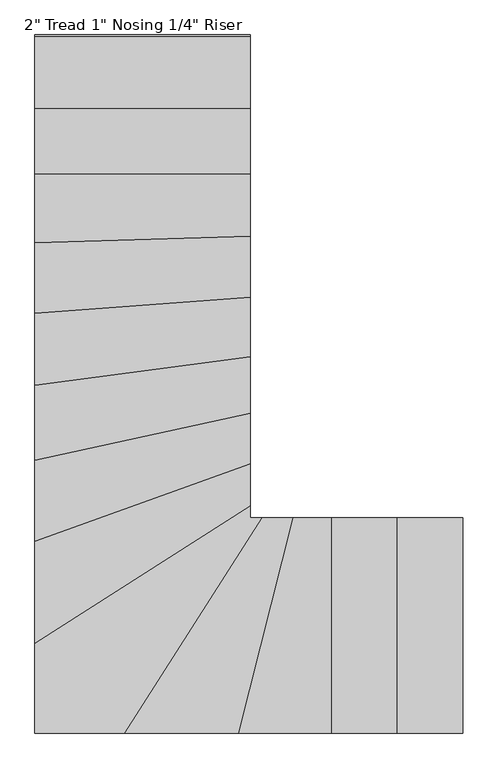
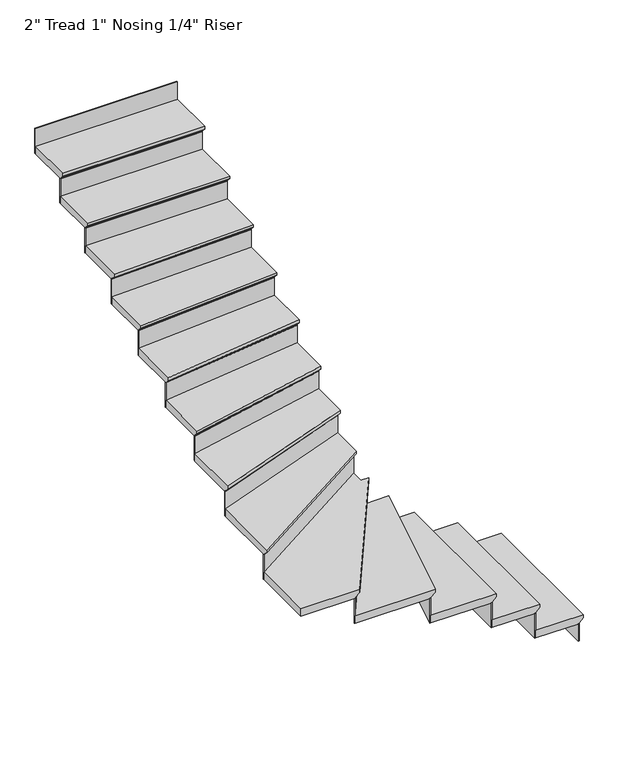
"""IFC4 building model written with IfcOpenShell, lengths in millimetres: stair flight geometry."""

from ifc_helpers import new_model, si_unit, origin, place, context, project, spatial, faceted_brep, source, transform, mapped, element, save


def stair_flight_d75d4b7d(model_context):
    return source(origin(), model_context, "Body", "Brep", [
        faceted_brep([(-4378.4230036, -1246.1564015, 4028.0166667), (-4378.4230036, -1246.1564015, 4047.0666667), (-4378.4230036, -2160.5564015, 4047.0666667), (-4378.4230036, -2160.5564015, 4028.0166667), (-4403.8230036, -1246.1564015, 4002.6166667), (-4403.8230036, -2160.5564015, 4002.6166667), (-4683.2230036, -1246.1564015, 4047.0666667), (-4683.2230036, -2160.5564015, 4047.0666667), (-4403.8230036, -2160.5564015, 3996.2666667), (-4683.2230036, -2160.5564015, 3996.2666667), (-4683.2230036, -1246.1564015, 3996.2666667), (-4403.8230036, -1246.1564015, 3996.2666667)], [[[0, 1, 2, 3]], [[4, 0, 3, 5]], [[2, 1, 6, 7]], [[8, 9, 10, 11]], [[2, 7, 9, 8, 5, 3]], [[8, 11, 4, 5]], [[6, 1, 0, 4, 11, 10]], [[7, 6, 10, 9]]]),
        faceted_brep([(-4403.8230036, -1246.1564015, 3996.2666667), (-4403.8230036, -1246.1564015, 3877.7333333), (-4410.1730036, -1246.1564015, 3877.7333333), (-4410.1730036, -1246.1564015, 3996.2666667), (-4403.8230036, -2160.5564015, 3996.2666667), (-4410.1730036, -2160.5564015, 3996.2666667), (-4410.1730036, -2160.5564015, 3877.7333333), (-4403.8230036, -2160.5564015, 3877.7333333)], [[[0, 1, 2, 3]], [[4, 5, 6, 7]], [[1, 0, 4, 7]], [[2, 1, 7, 6]], [[3, 2, 6, 5]], [[0, 3, 5, 4]]]),
        faceted_brep([(-4683.2230036, -1246.1564015, 4165.6), (-4683.2230036, -1246.1564015, 3996.2666667), (-4689.5730036, -1246.1564015, 3996.2666667), (-4689.5730036, -1246.1564015, 4165.6), (-4683.2230036, -2160.5564015, 4165.6), (-4689.5730036, -2160.5564015, 4165.6), (-4689.5730036, -2160.5564015, 3996.2666667), (-4683.2230036, -2160.5564015, 3996.2666667)], [[[0, 1, 2, 3]], [[4, 5, 6, 7]], [[1, 0, 4, 7]], [[2, 1, 7, 6]], [[3, 2, 6, 5]], [[0, 3, 5, 4]]]),
        faceted_brep([(-4657.8230036, -2160.5564015, 4216.4), (-4657.8230036, -1246.1564015, 4216.4), (-4962.6230036, -1246.1564015, 4216.4), (-4962.6230036, -2160.5564015, 4216.4), (-4683.2230036, -2160.5564015, 4165.6), (-4962.6230036, -2160.5564015, 4165.6), (-4962.6230036, -1246.1564015, 4165.6), (-4683.2230036, -1246.1564015, 4165.6), (-4683.2230036, -2160.5564015, 4171.95), (-4657.8230036, -2160.5564015, 4197.35), (-4683.2230036, -1246.1564015, 4171.95), (-4657.8230036, -1246.1564015, 4197.35)], [[[0, 1, 2, 3]], [[4, 5, 6, 7]], [[0, 3, 5, 4, 8, 9]], [[4, 7, 10, 8]], [[2, 1, 11, 10, 7, 6]], [[3, 2, 6, 5]], [[11, 1, 0, 9]], [[10, 11, 9, 8]]]),
        faceted_brep([(-4962.6230036, -1246.1564015, 4334.9333333), (-4962.6230036, -1246.1564015, 4165.6), (-4968.9730036, -1246.1564015, 4165.6), (-4968.9730036, -1246.1564015, 4334.9333333), (-4962.6230036, -2160.5564015, 4334.9333333), (-4968.9730036, -2160.5564015, 4334.9333333), (-4968.9730036, -2160.5564015, 4165.6), (-4962.6230036, -2160.5564015, 4165.6)], [[[0, 1, 2, 3]], [[4, 5, 6, 7]], [[1, 0, 4, 7]], [[2, 1, 7, 6]], [[3, 2, 6, 5]], [[0, 3, 5, 4]]]),
        faceted_brep([(-4937.2230036, -2160.5564015, 4385.7333333), (-4937.2230036, -1246.1564015, 4385.7333333), (-5127.3280374, -1246.1564015, 4385.7333333), (-5358.313714, -2160.5564015, 4385.7333333), (-4962.6230036, -2160.5564015, 4334.9333333), (-5358.313714, -2160.5564015, 4334.9333333), (-5127.3280374, -1246.1564015, 4334.9333333), (-4962.6230036, -1246.1564015, 4334.9333333), (-4962.6230036, -2160.5564015, 4341.2833333), (-4937.2230036, -2160.5564015, 4366.6833333), (-4962.6230036, -1246.1564015, 4341.2833333), (-4937.2230036, -1246.1564015, 4366.6833333)], [[[0, 1, 2, 3]], [[4, 5, 6, 7]], [[0, 3, 5, 4, 8, 9]], [[4, 7, 10, 8]], [[2, 1, 11, 10, 7, 6]], [[3, 2, 6, 5]], [[11, 1, 0, 9]], [[10, 11, 9, 8]]]),
        faceted_brep([(-5127.3280374, -1246.1564015, 4504.2666667), (-5127.3280374, -1246.1564015, 4334.9333333), (-5133.8775055, -1246.1564015, 4334.9333333), (-5133.8775055, -1246.1564015, 4504.2666667), (-5358.313714, -2160.5564015, 4504.2666667), (-5364.8631821, -2160.5564015, 4504.2666667), (-5364.8631821, -2160.5564015, 4334.9333333), (-5358.313714, -2160.5564015, 4334.9333333)], [[[0, 1, 2, 3]], [[4, 5, 6, 7]], [[1, 0, 4, 7]], [[2, 1, 7, 6]], [[3, 2, 6, 5]], [[0, 3, 5, 4]]]),
        faceted_brep([(-5332.1158419, -2160.5564015, 4555.0666667), (-5101.1301653, -1246.1564015, 4555.0666667), (-5261.5956265, -1246.1564015, 4555.0666667), (-5846.1950619, -2160.5564015, 4555.0666667), (-5358.313714, -2160.5564015, 4504.2666667), (-5846.1950619, -2160.5564015, 4504.2666667), (-5261.5956265, -1246.1564015, 4504.2666667), (-5127.3280374, -1246.1564015, 4504.2666667), (-5358.313714, -2160.5564015, 4510.6166667), (-5332.1158419, -2160.5564015, 4536.0166667), (-5127.3280374, -1246.1564015, 4510.6166667), (-5101.1301653, -1246.1564015, 4536.0166667)], [[[0, 1, 2, 3]], [[4, 5, 6, 7]], [[0, 3, 5, 4, 8, 9]], [[4, 7, 10, 8]], [[2, 1, 11, 10, 7, 6]], [[3, 2, 6, 5]], [[11, 1, 0, 9]], [[10, 11, 9, 8]]]),
        faceted_brep([(-5261.5956265, -1246.1564015, 4673.6), (-5261.5956265, -1246.1564015, 4504.2666667), (-5269.1324569, -1246.1564015, 4504.2666667), (-5269.1324569, -1246.1564015, 4673.6), (-5846.1950619, -2160.5564015, 4673.6), (-5853.7318923, -2160.5564015, 4673.6), (-5853.7318923, -2160.5564015, 4504.2666667), (-5846.1950619, -2160.5564015, 4504.2666667)], [[[0, 1, 2, 3]], [[4, 5, 6, 7]], [[1, 0, 4, 7]], [[2, 1, 7, 6]], [[3, 2, 6, 5]], [[0, 3, 5, 4]]]),
        faceted_brep([(-6196.7599931, -1749.696827, 4724.4), (-6196.7599931, -2160.5564015, 4724.4), (-5816.0477402, -2160.5564015, 4724.4), (-5231.4483048, -1246.1564015, 4724.4), (-5282.3599931, -1246.1564015, 4724.4), (-5282.3599931, -1165.0973916, 4724.4), (-6196.7599931, -2160.5564015, 4673.6), (-6196.7599931, -1749.696827, 4673.6), (-5282.3599931, -1165.0973916, 4673.6), (-5282.3599931, -1246.1564015, 4673.6), (-5261.5956265, -1246.1564015, 4673.6), (-5846.1950619, -2160.5564015, 4673.6), (-5261.5956265, -1246.1564015, 4679.95), (-5846.1950619, -2160.5564015, 4679.95), (-5231.4483048, -1246.1564015, 4705.35), (-5816.0477402, -2160.5564015, 4705.35)], [[[0, 1, 2, 3, 4, 5]], [[6, 7, 8, 9, 10, 11]], [[1, 0, 7, 6]], [[11, 10, 12, 13]], [[4, 3, 14, 12, 10, 9]], [[0, 5, 8, 7]], [[14, 3, 2, 15]], [[12, 14, 15, 13]], [[2, 1, 6, 11, 13, 15]], [[5, 4, 9, 8]]]),
        faceted_brep([(-5282.3599931, -1165.0973916, 4842.9333333), (-5282.3599931, -1165.0973916, 4673.6), (-5282.3599931, -1157.5605612, 4673.6), (-5282.3599931, -1157.5605612, 4842.9333333), (-6196.7599931, -1749.696827, 4842.9333333), (-6196.7599931, -1742.1599966, 4842.9333333), (-6196.7599931, -1742.1599966, 4673.6), (-6196.7599931, -1749.696827, 4673.6)], [[[0, 1, 2, 3]], [[4, 5, 6, 7]], [[1, 0, 4, 7]], [[2, 1, 7, 6]], [[3, 2, 6, 5]], [[0, 3, 5, 4]]]),
        faceted_brep([(-6196.7599931, -1779.8441487, 4893.7333333), (-5282.3599931, -1195.2447133, 4893.7333333), (-5282.3599931, -989.1410797, 4893.7333333), (-6196.7599931, -1317.7175845, 4893.7333333), (-6196.7599931, -1749.696827, 4842.9333333), (-6196.7599931, -1317.7175845, 4842.9333333), (-5282.3599931, -989.1410797, 4842.9333333), (-5282.3599931, -1165.0973916, 4842.9333333), (-6196.7599931, -1749.696827, 4849.2833333), (-6196.7599931, -1779.8441487, 4874.6833333), (-5282.3599931, -1165.0973916, 4849.2833333), (-5282.3599931, -1195.2447133, 4874.6833333)], [[[0, 1, 2, 3]], [[4, 5, 6, 7]], [[0, 3, 5, 4, 8, 9]], [[4, 7, 10, 8]], [[2, 1, 11, 10, 7, 6]], [[3, 2, 6, 5]], [[11, 1, 0, 9]], [[10, 11, 9, 8]]]),
        faceted_brep([(-5282.3599931, -989.1410797, 5012.2666667), (-5282.3599931, -989.1410797, 4842.9333333), (-5282.3599931, -982.3935597, 4842.9333333), (-5282.3599931, -982.3935597, 5012.2666667), (-6196.7599931, -1317.7175845, 5012.2666667), (-6196.7599931, -1310.9700645, 5012.2666667), (-6196.7599931, -1310.9700645, 4842.9333333), (-6196.7599931, -1317.7175845, 4842.9333333)], [[[0, 1, 2, 3]], [[4, 5, 6, 7]], [[1, 0, 4, 7]], [[2, 1, 7, 6]], [[3, 2, 6, 5]], [[0, 3, 5, 4]]]),
        faceted_brep([(-6196.7599931, -1344.7076644, 5063.0666667), (-5282.3599931, -1016.1311596, 5063.0666667), (-5282.3599931, -775.0246806, 5063.0666667), (-6196.7599931, -975.0133472, 5063.0666667), (-6196.7599931, -1317.7175845, 5012.2666667), (-6196.7599931, -975.0133472, 5012.2666667), (-5282.3599931, -775.0246806, 5012.2666667), (-5282.3599931, -989.1410797, 5012.2666667), (-6196.7599931, -1317.7175845, 5018.6166667), (-6196.7599931, -1344.7076644, 5044.0166667), (-5282.3599931, -989.1410797, 5018.6166667), (-5282.3599931, -1016.1311596, 5044.0166667)], [[[0, 1, 2, 3]], [[4, 5, 6, 7]], [[0, 3, 5, 4, 8, 9]], [[4, 7, 10, 8]], [[2, 1, 11, 10, 7, 6]], [[3, 2, 6, 5]], [[11, 1, 0, 9]], [[10, 11, 9, 8]]]),
        faceted_brep([(-5282.3599931, -775.0246806, 5181.6), (-5282.3599931, -775.0246806, 5012.2666667), (-5282.3599931, -768.5245811, 5012.2666667), (-5282.3599931, -768.5245811, 5181.6), (-6196.7599931, -975.0133472, 5181.6), (-6196.7599931, -968.5132477, 5181.6), (-6196.7599931, -968.5132477, 5012.2666667), (-6196.7599931, -975.0133472, 5012.2666667)], [[[0, 1, 2, 3]], [[4, 5, 6, 7]], [[1, 0, 4, 7]], [[2, 1, 7, 6]], [[3, 2, 6, 5]], [[0, 3, 5, 4]]]),
        faceted_brep([(-6196.7599931, -1001.0137453, 5232.4), (-5282.3599931, -801.0250787, 5232.4), (-5282.3599931, -535.4776405, 5232.4), (-6196.7599931, -656.5180526, 5232.4), (-6196.7599931, -975.0133472, 5181.6), (-6196.7599931, -656.5180526, 5181.6), (-5282.3599931, -535.4776405, 5181.6), (-5282.3599931, -775.0246806, 5181.6), (-6196.7599931, -975.0133472, 5187.95), (-6196.7599931, -1001.0137453, 5213.35), (-5282.3599931, -775.0246806, 5187.95), (-5282.3599931, -801.0250787, 5213.35)], [[[0, 1, 2, 3]], [[4, 5, 6, 7]], [[0, 3, 5, 4, 8, 9]], [[4, 7, 10, 8]], [[2, 1, 11, 10, 7, 6]], [[3, 2, 6, 5]], [[11, 1, 0, 9]], [[10, 11, 9, 8]]]),
        faceted_brep([(-5282.3599931, -535.4776405, 5350.9333333), (-5282.3599931, -535.4776405, 5181.6), (-5282.3599931, -529.0722492, 5181.6), (-5282.3599931, -529.0722492, 5350.9333333), (-6196.7599931, -656.5180526, 5350.9333333), (-6196.7599931, -650.1126613, 5350.9333333), (-6196.7599931, -650.1126613, 5181.6), (-6196.7599931, -656.5180526, 5181.6)], [[[0, 1, 2, 3]], [[4, 5, 6, 7]], [[1, 0, 4, 7]], [[2, 1, 7, 6]], [[3, 2, 6, 5]], [[0, 3, 5, 4]]]),
        faceted_brep([(-6196.7599931, -682.139618, 5401.7333333), (-5282.3599931, -561.099206, 5401.7333333), (-5282.3599931, -282.9309158, 5401.7333333), (-6196.7599931, -350.56912, 5401.7333333), (-6196.7599931, -656.5180526, 5350.9333333), (-6196.7599931, -350.56912, 5350.9333333), (-5282.3599931, -282.9309158, 5350.9333333), (-5282.3599931, -535.4776405, 5350.9333333), (-6196.7599931, -656.5180526, 5357.2833333), (-6196.7599931, -682.139618, 5382.6833333), (-5282.3599931, -535.4776405, 5357.2833333), (-5282.3599931, -561.099206, 5382.6833333)], [[[0, 1, 2, 3]], [[4, 5, 6, 7]], [[0, 3, 5, 4, 8, 9]], [[4, 7, 10, 8]], [[2, 1, 11, 10, 7, 6]], [[3, 2, 6, 5]], [[11, 1, 0, 9]], [[10, 11, 9, 8]]]),
        faceted_brep([(-5282.3599931, -282.9309158, 5520.2666667), (-5282.3599931, -282.9309158, 5350.9333333), (-5282.3599931, -276.5635673, 5350.9333333), (-5282.3599931, -276.5635673, 5520.2666667), (-6196.7599931, -350.56912, 5520.2666667), (-6196.7599931, -344.2017715, 5520.2666667), (-6196.7599931, -344.2017715, 5350.9333333), (-6196.7599931, -350.56912, 5350.9333333)], [[[0, 1, 2, 3]], [[4, 5, 6, 7]], [[1, 0, 4, 7]], [[2, 1, 7, 6]], [[3, 2, 6, 5]], [[0, 3, 5, 4]]]),
        faceted_brep([(-6196.7599931, -376.0385141, 5571.0666667), (-5282.3599931, -308.4003099, 5571.0666667), (-5282.3599931, -22.8518026, 5571.0666667), (-6196.7599931, -51.9612867, 5571.0666667), (-6196.7599931, -350.56912, 5520.2666667), (-6196.7599931, -51.9612867, 5520.2666667), (-5282.3599931, -22.8518026, 5520.2666667), (-5282.3599931, -282.9309158, 5520.2666667), (-6196.7599931, -350.56912, 5526.6166667), (-6196.7599931, -376.0385141, 5552.0166667), (-5282.3599931, -282.9309158, 5526.6166667), (-5282.3599931, -308.4003099, 5552.0166667)], [[[0, 1, 2, 3]], [[4, 5, 6, 7]], [[0, 3, 5, 4, 8, 9]], [[4, 7, 10, 8]], [[2, 1, 11, 10, 7, 6]], [[3, 2, 6, 5]], [[11, 1, 0, 9]], [[10, 11, 9, 8]]]),
        faceted_brep([(-5282.3599931, -22.8518026, 5689.6), (-5282.3599931, -22.8518026, 5520.2666667), (-5282.3599931, -16.4985857, 5520.2666667), (-5282.3599931, -16.4985857, 5689.6), (-6196.7599931, -51.9612867, 5689.6), (-6196.7599931, -45.6080698, 5689.6), (-6196.7599931, -45.6080698, 5520.2666667), (-6196.7599931, -51.9612867, 5520.2666667)], [[[0, 1, 2, 3]], [[4, 5, 6, 7]], [[1, 0, 4, 7]], [[2, 1, 7, 6]], [[3, 2, 6, 5]], [[0, 3, 5, 4]]]),
        faceted_brep([(-6196.7599931, -77.3741541, 5740.4), (-5282.3599931, -48.26467, 5740.4), (-5282.3599931, 241.980588, 5740.4), (-6196.7599931, 241.980588, 5740.4), (-6196.7599931, -51.9612867, 5689.6), (-6196.7599931, 241.980588, 5689.6), (-5282.3599931, 241.980588, 5689.6), (-5282.3599931, -22.8518026, 5689.6), (-6196.7599931, -51.9612867, 5695.95), (-6196.7599931, -77.3741541, 5721.35), (-5282.3599931, -22.8518026, 5695.95), (-5282.3599931, -48.26467, 5721.35)], [[[0, 1, 2, 3]], [[4, 5, 6, 7]], [[0, 3, 5, 4, 8, 9]], [[4, 7, 10, 8]], [[2, 1, 11, 10, 7, 6]], [[3, 2, 6, 5]], [[11, 1, 0, 9]], [[10, 11, 9, 8]]]),
        faceted_brep([(-5282.3599931, 241.980588, 5858.9333333), (-5282.3599931, 241.980588, 5689.6), (-5282.3599931, 248.330588, 5689.6), (-5282.3599931, 248.330588, 5858.9333333), (-6196.7599931, 241.980588, 5858.9333333), (-6196.7599931, 248.330588, 5858.9333333), (-6196.7599931, 248.330588, 5689.6), (-6196.7599931, 241.980588, 5689.6)], [[[0, 1, 2, 3]], [[4, 5, 6, 7]], [[1, 0, 4, 7]], [[2, 1, 7, 6]], [[3, 2, 6, 5]], [[0, 3, 5, 4]]]),
        faceted_brep([(-6196.7599931, 216.580588, 5909.7333333), (-5282.3599931, 216.580588, 5909.7333333), (-5282.3599931, 521.380588, 5909.7333333), (-6196.7599931, 521.380588, 5909.7333333), (-6196.7599931, 241.980588, 5858.9333333), (-6196.7599931, 521.380588, 5858.9333333), (-5282.3599931, 521.380588, 5858.9333333), (-5282.3599931, 241.980588, 5858.9333333), (-6196.7599931, 241.980588, 5865.2833333), (-6196.7599931, 216.580588, 5890.6833333), (-5282.3599931, 241.980588, 5865.2833333), (-5282.3599931, 216.580588, 5890.6833333)], [[[0, 1, 2, 3]], [[4, 5, 6, 7]], [[0, 3, 5, 4, 8, 9]], [[4, 7, 10, 8]], [[2, 1, 11, 10, 7, 6]], [[3, 2, 6, 5]], [[11, 1, 0, 9]], [[10, 11, 9, 8]]]),
        faceted_brep([(-5282.3599931, 521.380588, 6028.2666667), (-5282.3599931, 521.380588, 5858.9333333), (-5282.3599931, 527.730588, 5858.9333333), (-5282.3599931, 527.730588, 6028.2666667), (-6196.7599931, 521.380588, 6028.2666667), (-6196.7599931, 527.730588, 6028.2666667), (-6196.7599931, 527.730588, 5858.9333333), (-6196.7599931, 521.380588, 5858.9333333)], [[[0, 1, 2, 3]], [[4, 5, 6, 7]], [[1, 0, 4, 7]], [[2, 1, 7, 6]], [[3, 2, 6, 5]], [[0, 3, 5, 4]]]),
        faceted_brep([(-5282.3599931, 800.780588, 6197.6), (-5282.3599931, 800.780588, 6028.2666667), (-5282.3599931, 807.130588, 6028.2666667), (-5282.3599931, 807.130588, 6197.6), (-6196.7599931, 800.780588, 6197.6), (-6196.7599931, 807.130588, 6197.6), (-6196.7599931, 807.130588, 6028.2666667), (-6196.7599931, 800.780588, 6028.2666667)], [[[0, 1, 2, 3]], [[4, 5, 6, 7]], [[1, 0, 4, 7]], [[2, 1, 7, 6]], [[3, 2, 6, 5]], [[0, 3, 5, 4]]]),
        faceted_brep([(-6196.7599931, 495.980588, 6079.0666667), (-5282.3599931, 495.980588, 6079.0666667), (-5282.3599931, 800.780588, 6079.0666667), (-6196.7599931, 800.780588, 6079.0666667), (-6196.7599931, 521.380588, 6028.2666667), (-6196.7599931, 800.780588, 6028.2666667), (-5282.3599931, 800.780588, 6028.2666667), (-5282.3599931, 521.380588, 6028.2666667), (-6196.7599931, 521.380588, 6034.6166667), (-6196.7599931, 495.980588, 6060.0166667), (-5282.3599931, 521.380588, 6034.6166667), (-5282.3599931, 495.980588, 6060.0166667)], [[[0, 1, 2, 3]], [[4, 5, 6, 7]], [[0, 3, 5, 4, 8, 9]], [[4, 7, 10, 8]], [[2, 1, 11, 10, 7, 6]], [[3, 2, 6, 5]], [[11, 1, 0, 9]], [[10, 11, 9, 8]]]),
    ])


if __name__ == "__main__":
    model = new_model("IFC4")
    model_context = context("Model", 3, world=origin())
    ifc_project = project(units=[si_unit("LENGTHUNIT", "METRE", prefix="MILLI")], contexts=[model_context])
    site = spatial("IfcSite", under=ifc_project)
    building = spatial("IfcBuilding", under=site)
    placement = place(None, origin())
    stair_flight_shape = stair_flight_d75d4b7d(model_context)
    element("IfcStairFlight", 1, ObjectType="2\" Tread 1\" Nosing 1/4\" Riser", at=placement, inside=building, context=model_context, shape_type="MappedRepresentation", body=[
        mapped(stair_flight_shape, transform((0.0, 0.0, 0.0), x_axis=(1.0, 0.0, 0.0), y_axis=(0.0, 1.0, 0.0), z_axis=(0.0, 0.0, 1.0))),
    ])
    save(model, "model.ifc")
